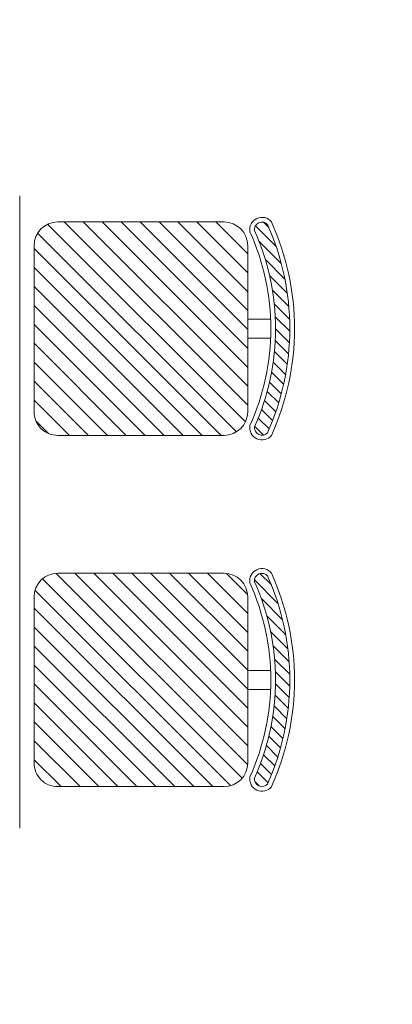
# Model space of a CAD drawing. Units: inches. Extents: x 375 to 1122, y 27 to 1069.
# Tile 65 of 155: x 747 to 774, y 253 to 326. Entities that reach past the tile are written whole.
import ezdxf

# ---------------------------------------------------------------- set-up
doc = ezdxf.new("R2010")
doc.units = ezdxf.units.IN
doc.layers.add('A-ANNO-DIMS', color=2, linetype='Continuous', lineweight=18)
doc.layers.add('Furniture', color=30, linetype='Continuous', lineweight=18)
doc.styles.get("Standard").update_dxf_attribs({"font": 'arial.ttf'})
doc.dimstyles.new('ISO-25', dxfattribs={"dimtxt": 12, "dimasz": 2.5, "dimexe": 1.5, "dimexo": 1.5, "dimtad": 1, "dimdec": 1, "dimlunit": 3, "dimtxsty": 'Standard', "dimblk": 'ARCHTICK', "dimcen": 2.5, "dimadec": 0, "dimazin": 0, "dimtfac": 1, "dimtdec": 1, "dimtmove": 0, "dimatfit": 3, "dimfxl": 1.5, "dimfxlon": 1, "dimarcsym": 0})

# ---------------------------------------------------------------- blocks, each defined once
blk = doc.blocks.new('A$C403C54AD')
at = {"ltscale": 0.05}
for p, q in [((1.0628, 2.0477, -0.0006), (1.0346, 2.0195, -0.0006)), ((1.0849, 2.048, -0.0006), (1.0582, 2.0213, -0.0006)), ((1.106, 2.0473, -0.0006), (1.0805, 2.0219, -0.0006)), ((1.716, 2.0479, -0.0006), (1.6883, 2.0202, -0.0006)), ((1.7378, 2.0479, -0.0006), (1.7115, 2.0216, -0.0006)), ((0.9605, 2.0325, -0.0006), (0.9198, 1.9918, -0.0006)), ((0.9888, 2.039, -0.0006), (0.953, 2.0032, -0.0006)), ((1.015, 2.0435, -0.0006), (0.9825, 2.0109, -0.0006)), ((1.0396, 2.0463, -0.0006), (1.0095, 2.0162, -0.0006)), ((1.1262, 2.0458, -0.0006), (1.1017, 2.0213, -0.0006)), ((1.1456, 2.0435, -0.0006), (1.122, 2.0199, -0.0006)), ((1.1643, 2.0404, -0.0006), (1.1415, 2.0176, -0.0006)), ((1.1824, 2.0368, -0.0006), (1.1603, 2.0146, -0.0006)), ((1.1999, 2.0325, -0.0006), (1.1783, 2.0108, -0.0006)), ((1.6158, 2.0348, -0.0006), (1.5768, 1.9958, -0.0006)), ((1.6434, 2.0406, -0.0006), (1.6087, 2.0059, -0.0006)), ((1.6691, 2.0445, -0.0006), (1.6374, 2.0128, -0.0006)), ((1.6932, 2.0469, -0.0006), (1.6637, 2.0174, -0.0006)), ((1.7586, 2.0469, -0.0006), (1.7335, 2.0218, -0.0006)), ((1.7786, 2.0451, -0.0006), (1.7544, 2.021, -0.0006)), ((1.7978, 2.0426, -0.0006), (1.7744, 2.0193, -0.0006)), ((1.8163, 2.0394, -0.0006), (1.7937, 2.0167, -0.0006)), ((1.8342, 2.0355, -0.0006), (1.8122, 2.0135, -0.0006)), ((1.8515, 2.0311, -0.0006), (1.8301, 2.0096, -0.0006)), ((0.9293, 2.0231, -0.0006), (0.8911, 1.9849, -0.0006)), ((1.2169, 2.0277, -0.0006), (1.1957, 2.0065, -0.0006)), ((1.2333, 2.0223, -0.0006), (1.2126, 2.0016, -0.0006)), ((1.2493, 2.0165, -0.0006), (1.2289, 1.9961, -0.0006)), ((1.5517, 2.0142, -0.0006), (1.5308, 1.9933, -0.0006)), ((1.5856, 2.0264, -0.0006), (1.5425, 1.9832, -0.0006)), ((1.8683, 2.0261, -0.0006), (1.8473, 2.0051, -0.0006)), ((1.8846, 2.0206, -0.0006), (1.864, 2, -0.0006)), ((1.9004, 2.0146, -0.0006), (1.8801, 1.9943, -0.0006)), ((0.8939, 2.0094, -0.0006), (0.8844, 1.9999, -0.0006)), ((1.2647, 2.0102, -0.0006), (1.2447, 1.9902, -0.0006)), ((1.2759, 1.9996, -0.0006), (1.26, 1.9837, -0.0006)), ((1.9157, 2.0082, -0.0006), (1.8958, 1.9882, -0.0006)), ((1.9217, 1.9924, -0.0006), (1.9133, 1.9839, -0.0006)), ((1.2211, 1.9709, -0.0006), (0.8839, 1.6337, -0.0006)), ((1.1862, 1.9709, -0.0006), (0.8839, 1.6685, -0.0006)), ((1.1514, 1.9709, -0.0006), (0.8839, 1.7033, -0.0006)), ((1.1166, 1.9709, -0.0006), (0.8839, 1.7382, -0.0006)), ((1.0818, 1.9709, -0.0006), (0.8839, 1.773, -0.0006)), ((1.0469, 1.9709, -0.0006), (0.8839, 1.8078, -0.0006)), ((1.0121, 1.9709, -0.0006), (0.8839, 1.8427, -0.0006)), ((0.9773, 1.9709, -0.0006), (0.8839, 1.8775, -0.0006)), ((0.9424, 1.9709, -0.0006), (0.8839, 1.9123, -0.0006)), ((1.2517, 1.9667, -0.0006), (0.8881, 1.6031, -0.0006)), ((1.848, 1.9709, -0.0006), (1.5302, 1.6531, -0.0006)), ((1.8131, 1.9709, -0.0006), (1.5302, 1.6879, -0.0006)), ((1.7783, 1.9709, -0.0006), (1.5302, 1.7228, -0.0006)), ((1.7435, 1.9709, -0.0006), (1.5302, 1.7576, -0.0006)), ((1.7087, 1.9709, -0.0006), (1.5302, 1.7924, -0.0006)), ((1.6738, 1.9709, -0.0006), (1.5302, 1.8272, -0.0006)), ((1.639, 1.9709, -0.0006), (1.5302, 1.8621, -0.0006)), ((1.6042, 1.9709, -0.0006), (1.5302, 1.8969, -0.0006)), ((1.8827, 1.9708, -0.0006), (1.5303, 1.6184, -0.0006)), ((1.5691, 1.9706, -0.0006), (1.5304, 1.932, -0.0006)), ((1.9073, 1.9606, -0.0006), (1.5405, 1.5937, -0.0006)), ((1.27, 1.9502, -0.0006), (0.9046, 1.5847, -0.0006)), ((1.9211, 1.9395, -0.0006), (1.5615, 1.58, -0.0006)), ((1.2765, 1.9219, -0.0006), (0.9329, 1.5782, -0.0006)), ((1.9228, 1.9065, -0.0006), (1.5946, 1.5782, -0.0006)), ((1.2765, 1.8871, -0.0006), (0.9677, 1.5782, -0.0006)), ((1.9228, 1.8716, -0.0006), (1.6294, 1.5782, -0.0006)), ((1.2765, 1.8522, -0.0006), (1.0025, 1.5782, -0.0006)), ((1.9228, 1.8368, -0.0006), (1.6643, 1.5782, -0.0006)), ((1.2765, 1.8174, -0.0006), (1.0374, 1.5782, -0.0006)), ((1.9228, 1.802, -0.0006), (1.6991, 1.5782, -0.0006)), ((1.2765, 1.7826, -0.0006), (1.0722, 1.5782, -0.0006)), ((1.9228, 1.7671, -0.0006), (1.7339, 1.5782, -0.0006)), ((1.2765, 1.7477, -0.0006), (1.107, 1.5782, -0.0006)), ((1.9228, 1.7323, -0.0006), (1.7687, 1.5782, -0.0006)), ((1.2765, 1.7129, -0.0006), (1.1418, 1.5782, -0.0006)), ((1.9228, 1.6975, -0.0006), (1.8036, 1.5782, -0.0006)), ((1.2765, 1.6781, -0.0006), (1.1767, 1.5782, -0.0006)), ((1.9228, 1.6627, -0.0006), (1.8384, 1.5782, -0.0006)), ((1.2765, 1.6433, -0.0006), (1.2115, 1.5782, -0.0006)), ((1.9228, 1.6278, -0.0006), (1.8732, 1.5782, -0.0006)), ((1.2732, 1.6051, -0.0006), (1.2497, 1.5816, -0.0006))]:
    blk.add_line(p, q, dxfattribs=at)
for p, q in [((1.0628, 1.9709, -0.0006), (1.0628, 2.0131, -0.0006)), ((1.0977, 1.9709, -0.0006), (1.0977, 2.0131, -0.0006)), ((1.7091, 1.9709, -0.0006), (1.7091, 2.0131, -0.0006)), ((1.744, 1.9709, -0.0006), (1.744, 2.0131, -0.0006)), ((0.9275, 1.9709, -0.0006), (1.2329, 1.9709, -0.0006)), ((1.5738, 1.9709, -0.0006), (1.8792, 1.9709, -0.0006)), ((0.8839, 1.7527, -0.0006), (0.8839, 1.9273, -0.0006)), ((1.2765, 1.9273, -0.0006), (1.2765, 1.6218, -0.0006)), ((1.5302, 1.7527, -0.0006), (1.5302, 1.9273, -0.0006)), ((1.9228, 1.9273, -0.0006), (1.9228, 1.6218, -0.0006)), ((0.8839, 1.6218, -0.0006), (0.8839, 1.7527, -0.0006)), ((1.5302, 1.6218, -0.0006), (1.5302, 1.7527, -0.0006)), ((1.2329, 1.5782, -0.0006), (0.9275, 1.5782, -0.0006)), ((1.8792, 1.5782, -0.0006), (1.5738, 1.5782, -0.0006)), ((0.8357, 1.5519, -0.0006), (1.9992, 1.5519, -0.0006))]:
    blk.add_line(p, q)
for centre, radius, start, end in [((1.0802, 1.5793, -0.0006), 0.4774, 65.7176, 114.2824), ((1.0802, 1.5793, -0.0006), 0.4687, 65.7176, 114.2824), ((1.7265, 1.5793, -0.0006), 0.4774, 65.7176, 114.2824), ((1.7265, 1.5793, -0.0006), 0.4687, 65.7176, 114.2824), ((0.8978, 1.9969, -0.0006), 0.0225, 128.3306, 280.2342), ((1.0802, 1.5793, -0.0006), 0.4425, 65.7176, 114.2824), ((1.0802, 1.5793, -0.0006), 0.4338, 65.7176, 114.2824), ((1.2624, 1.997, -0.0006), 0.0225, 260.3316, 51.1036), ((1.5441, 1.9969, -0.0006), 0.0225, 128.3306, 280.2342), ((1.7265, 1.5793, -0.0006), 0.4425, 65.7176, 114.2824), ((1.7265, 1.5793, -0.0006), 0.4338, 65.7176, 114.2824), ((1.9087, 1.997, -0.0006), 0.0225, 260.3316, 51.1036), ((0.8978, 1.9969, -0.0006), 0.0138, 128.3306, 280.2342), ((1.2624, 1.997, -0.0006), 0.0138, 260.3316, 51.1036), ((1.5441, 1.9969, -0.0006), 0.0138, 128.3306, 280.2342), ((1.9087, 1.997, -0.0006), 0.0138, 260.3316, 51.1036), ((0.9275, 1.9273, -0.0006), 0.0436, 90, 180), ((1.2329, 1.9273, -0.0006), 0.0436, 0, 90), ((1.5738, 1.9273, -0.0006), 0.0436, 90, 180), ((1.8792, 1.9273, -0.0006), 0.0436, 0, 90), ((0.9275, 1.6218, -0.0006), 0.0436, 180, 270), ((1.2329, 1.6218, -0.0006), 0.0436, 270, 0), ((1.5738, 1.6218, -0.0006), 0.0436, 180, 270), ((1.8792, 1.6218, -0.0006), 0.0436, 270, 0)]:
    blk.add_arc(centre, radius, start, end)
blk = doc.blocks.new('_ArchTick')
at = {"color": 0, "linetype": 'ByBlock', "const_width": 0.15}
blk.add_lwpolyline([(-0.5, -0.5), (0.5, 0.5)], dxfattribs=at)
blk = doc.blocks.new('*D94')
at = {"layer": 'A-ANNO-DIMS', "color": 0, "lineweight": -2, "transparency": 16777216}
for p, q in [((734.007, 117.528), (734.007, 114.528)), ((773.007, 117.528), (773.007, 114.528)), ((734.007, 116.028), (773.007, 116.028))]:
    blk.add_line(p, q, dxfattribs=at)
at = {"layer": 'Defpoints', "color": 0, "transparency": 16777216}
for p in [(734.007, 667.528), (773.007, 667.528), (773.007, 116.028)]:
    blk.add_point(p, dxfattribs=at)
at = {"layer": 'A-ANNO-DIMS', "color": 0, "lineweight": -2, "transparency": 16777216, "xscale": 2.5, "yscale": 2.5, "zscale": 2.5, "rotation": 180}
blk.add_blockref('_ArchTick', (734.007, 116.028), dxfattribs=at)
at = {"layer": 'A-ANNO-DIMS', "color": 0, "lineweight": -2, "transparency": 16777216, "xscale": 2.5, "yscale": 2.5, "zscale": 2.5}
blk.add_blockref('_ArchTick', (773.007, 116.028), dxfattribs=at)
at = {"layer": 'A-ANNO-DIMS', "color": 0, "transparency": 16777216, "insert": (753.507, 122.784), "char_height": 12, "attachment_point": 5}
blk.add_mtext('3\'-3"', dxfattribs=at)

msp = doc.modelspace()

# ---------------------------------------------------------------- block references
at = {"layer": 'Furniture', "xscale": 39.9918517141215, "yscale": 39.9918517141215, "zscale": 39.9918517141215, "rotation": 270}
msp.add_blockref('A$C403C54AD', (684.955, 346.287, 0.024), dxfattribs=at)

# ---------------------------------------------------------------- dimensions: what is measured, and where the dimension line sits
at = {"layer": 'A-ANNO-DIMS'}
dim = msp.add_linear_dim(base=(773.007, 116.028), p1=(734.007, 667.528), p2=(773.007, 667.528), dimstyle='ISO-25', override={"dimdec": 1, "dimlfac": 1, "dimrnd": 0, "dimzin": 1, "dimdsep": 46, "dimlunit": 4, "dimfrac": 2}, dxfattribs=at)
dim.commit()
dim.dimension.update_dxf_attribs({"geometry": '*D94', "text_midpoint": (753.507, 122.784)})

doc.saveas('drawing.dxf')
